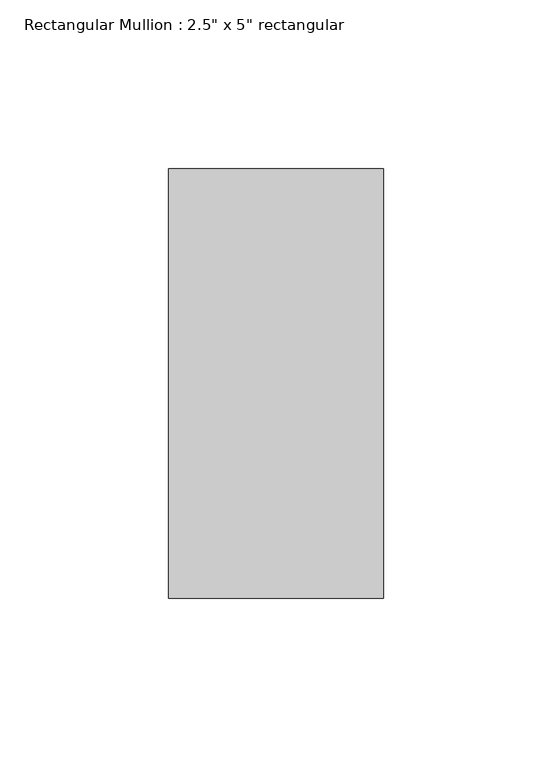
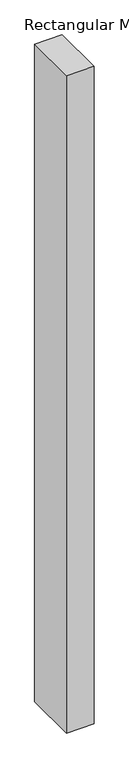
"""IFC4 building model written with IfcOpenShell, lengths in millimetres: member geometry."""

from ifc_helpers import new_model, si_unit, frame, origin, place, context, project, spatial, polyline, outline, extrude, source, transform, mapped, element, save


def member_2d77dfc0(model_context):
    return source(origin(), model_context, "Body", "SweptSolid", [
        extrude(outline(polyline([(31.75, 63.5), (31.75, -63.5), (-31.75, -63.5), (-31.75, 63.5), (31.75, 63.5)])), frame((0.0, 0.0, -1605.5835026), z_axis=(0.0, 0.0, 1.0), x_axis=(1.0, 0.0, 0.0)), (0.0, 0.0, 1.0), 1605.5835026),
    ])


if __name__ == "__main__":
    model = new_model("IFC4")
    model_context = context("Model", 3, world=origin())
    ifc_project = project(units=[si_unit("LENGTHUNIT", "METRE", prefix="MILLI")], contexts=[model_context])
    site = spatial("IfcSite", under=ifc_project)
    building = spatial("IfcBuilding", under=site)
    placement = place(None, origin())
    member_shape = member_2d77dfc0(model_context)
    element("IfcMember", 1, ObjectType="Rectangular Mullion : 2.5\" x 5\" rectangular", at=placement, inside=building, context=model_context, shape_type="MappedRepresentation", body=[
        mapped(member_shape, transform((0.0, 0.0, 0.0), x_axis=(1.0, 0.0, 0.0), y_axis=(0.0, 1.0, 0.0), z_axis=(0.0, 0.0, 1.0))),
    ])
    save(model, "model.ifc")

# Revit data of these elements
# Type "Rectangular Mullion : 2.5\" x 5\" rectangular"
#   built-in parameter 1007304 = 0.416667 (stored number, unit not read)
#   built-in parameter 1007301 = 0.104167 (stored number, unit not read)
#   built-in parameter 1007300 = 0.104167 (stored number, unit not read)
# Element 1 (IfcMember, "Rectangular Mullion : 2.5\" x 5\" rectangular")
#   Materials on its faces: "Aluminum"
# Materials
#   "Aluminum": class "Metal", colour RGB 247 247 247, transparency 0, Description = "Aluminum 6061", Cost = 0
